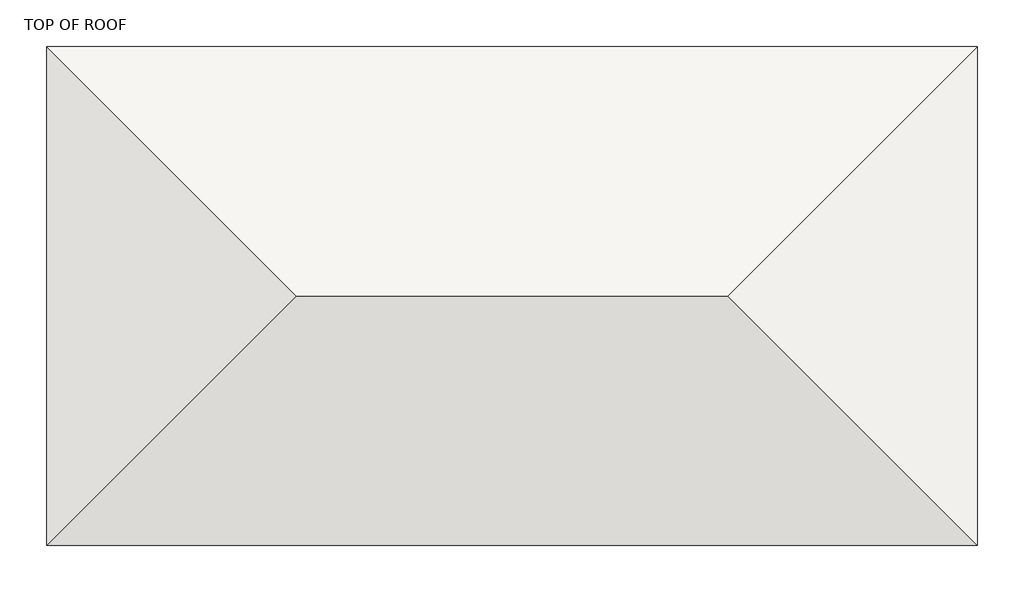
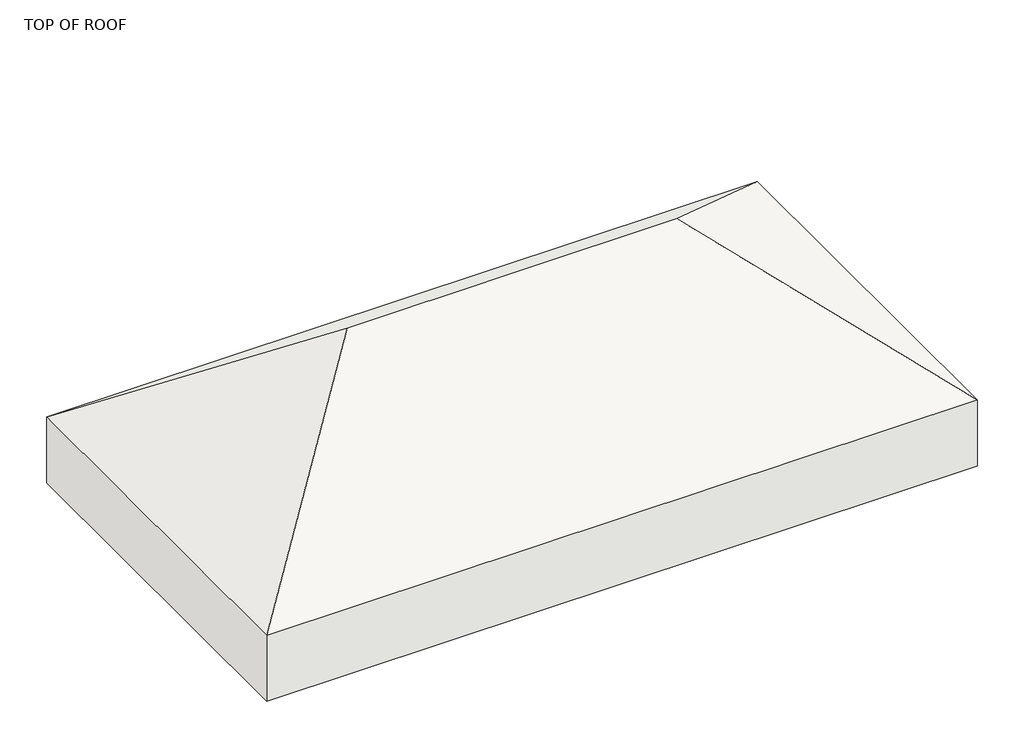
# One storey: 1 roof.
"""IFC4 building model written with IfcOpenShell, lengths in millimetres."""

from ifc_helpers import new_model, si_unit, origin, place, context, project, spatial, faceted_brep, element, save

model = new_model("IFC4")

# Units and contexts
model_context = context("Model", 3, world=origin())
ifc_project = project(units=[si_unit("LENGTHUNIT", "METRE", prefix="MILLI")], contexts=[model_context])

# Site, building, storey
site = spatial("IfcSite", under=ifc_project)
building = spatial("IfcBuilding", under=site)
storey = spatial("IfcBuildingStorey", under=building, Name="TOP OF ROOF", Elevation=20421.6)

# Roof
placement = place(None, origin())
element("IfcRoof", 1, ObjectType="Generic - 12\"", at=placement, inside=storey, context=model_context, shape_type="Brep", body=[
    faceted_brep([(-4881.5141359, 5016.1438161, 21202.7153132), (-5923.0012202, 6057.6309003, 20421.6), (-2038.3887202, 6057.6309003, 20421.6), (-3079.8758044, 5016.1438161, 21202.7153132), (-2038.3887202, 3974.6567318, 20421.6), (-5923.0012202, 3974.6567318, 20421.6), (-5923.0012202, 6057.6309003, 20802.6), (-4881.5141359, 5016.1438161, 21583.7153132), (-3079.8758044, 5016.1438161, 21583.7153132), (-2038.3887202, 6057.6309003, 20802.6), (-2038.3887202, 3974.6567318, 20802.6), (-5923.0012202, 3974.6567318, 20802.6)], [[[0, 1, 2, 3]], [[4, 3, 2]], [[5, 0, 3, 4]], [[1, 0, 5]], [[6, 7, 8, 9]], [[10, 9, 8]], [[11, 10, 8, 7]], [[6, 11, 7]], [[5, 11, 6, 1]], [[4, 10, 11, 5]], [[2, 9, 10, 4]], [[1, 6, 9, 2]]]),
])

save(model, "model.ifc")

# Revit data of these elements
# Type "Generic - 12\""
#   Assembly Code = "B1020"
#   Layers, outside or top first: 1' - 0" no material (function 1)
# Element 1 (IfcRoof, "Generic - 12\"")
#   built-in parameter 1001705 = 70.8127 (stored number, unit not read)
#   built-in parameter 1001710 = 33615
#   Phase Created = New Construction
#   Materials on its faces: "Default Roof"
# Materials
#   "Default Roof": colour RGB 88 101 114, transparency 0, Cost = 0
